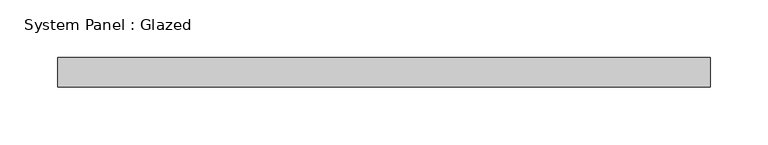
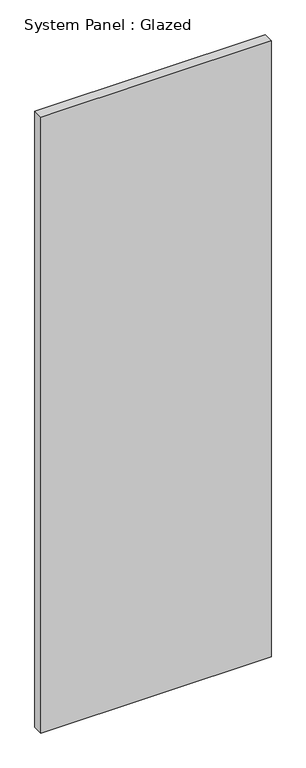
"""IFC4 building model written with IfcOpenShell, lengths in millimetres: plate geometry, System Panel : Glazed."""

from ifc_helpers import new_model, si_unit, origin, origin_with_axes, place, context, project, spatial, polyline, outline, extrude, source, transform, mapped, element, save


def system_panel_glazed_47f9b868(model_context):
    return source(origin(), model_context, "Body", "SweptSolid", [
        extrude(outline(polyline([(282.575, 19.05), (-282.575, 19.05), (-282.575, 44.45), (282.575, 44.45), (282.575, 19.05)])), origin_with_axes(), (0.0, 0.0, 1.0), 1598.9311114),
    ])


if __name__ == "__main__":
    model = new_model("IFC4")
    model_context = context("Model", 3, world=origin())
    ifc_project = project(units=[si_unit("LENGTHUNIT", "METRE", prefix="MILLI")], contexts=[model_context])
    site = spatial("IfcSite", under=ifc_project)
    building = spatial("IfcBuilding", under=site)
    placement = place(None, origin())
    system_panel_glazed_shape = system_panel_glazed_47f9b868(model_context)
    element("IfcPlate", 1, ObjectType="System Panel : Glazed", at=placement, inside=building, context=model_context, shape_type="MappedRepresentation", body=[
        mapped(system_panel_glazed_shape, transform((0.0, 0.0, 0.0), x_axis=(1.0, 0.0, 0.0), y_axis=(0.0, 1.0, 0.0), z_axis=(0.0, 0.0, 1.0))),
    ])
    save(model, "model.ifc")

# Revit data of these elements
# Type "System Panel : Glazed"
#   Construction Type Id = "GSP4R"
#   Analytic Construction = "1/8 in Pilkington single glazing"
#   Visual Light Transmittance = 0.9
#   Solar Heat Gain Coefficient = 0.86
#   Heat Transfer Coefficient (U) = 1.18115 BTU/(h·ft²·°F)
#   Define Thermal Properties by = 1
# Element 1 (IfcPlate, "System Panel : Glazed")
#   Materials on its faces: "Glass"
# Materials
#   "Glass": class "Glass", colour RGB 0 128 192, transparency 0.75, Description = "Soda Lime Glass", Cost = 0
